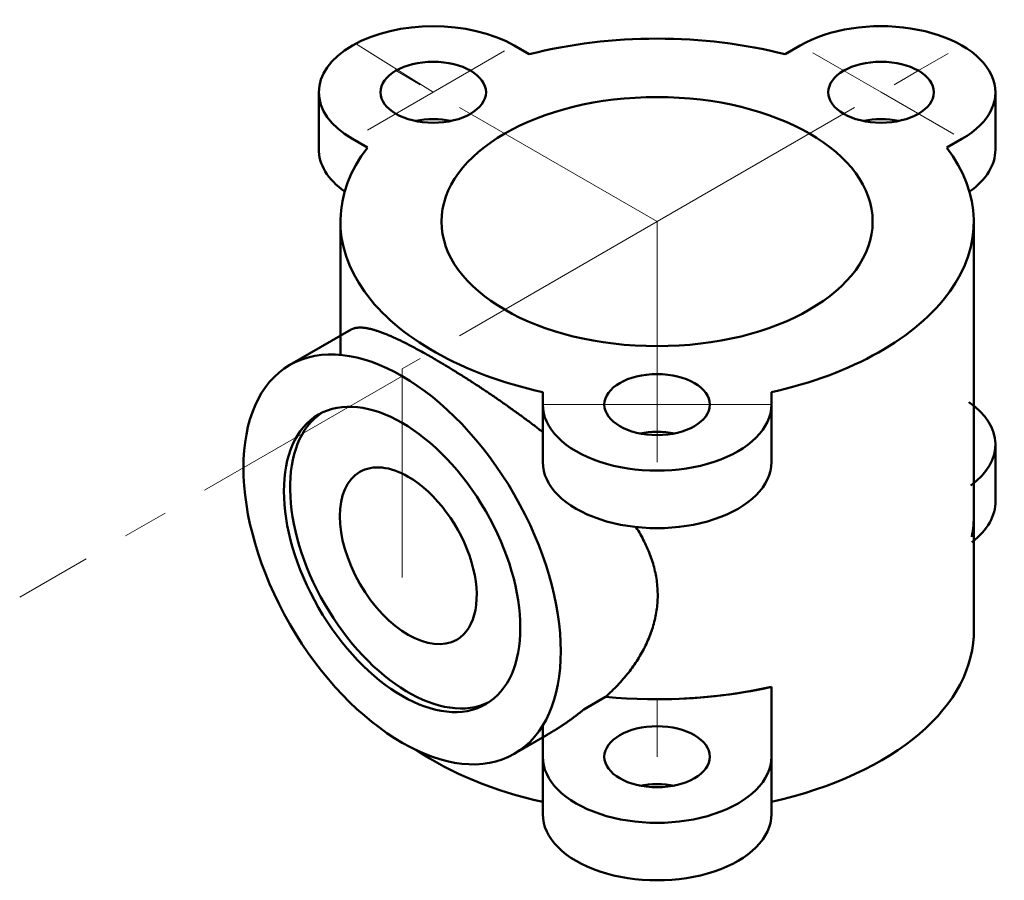
# Model space of a CAD drawing. Units: millimetres. Extents: x 3236 to 3373, y 1300 to 1420.
import ezdxf

# ---------------------------------------------------------------- set-up
doc = ezdxf.new("R2010")
doc.units = ezdxf.units.MM
doc.linetypes.add('CENTER', pattern=[50.8, 31.75, -6.35, 6.35, -6.35])
doc.layers.add('M-CNTR', color=4, linetype='CENTER', lineweight=18)
doc.layers.add('M-OUTL', color=7, linetype='Continuous', lineweight=50)

msp = doc.modelspace()

# ---------------------------------------------------------------- linework, layer by layer
at = {"layer": 'M-CNTR'}
for p, q in [((3293.15, 1409.64), (3282.35, 1416.4)), ((3293.15, 1409.64), (3303.09, 1415.38)), ((3355.5, 1409.64), (3346.02, 1415.11)), ((3360.7, 1412.64), (3364.83, 1415.03)), ((3324.32, 1391.64), (3287.95, 1412.64)), ((3324.32, 1391.64), (3360.7, 1412.64)), ((3293.15, 1409.64), (3283.99, 1404.35)), ((3355.5, 1409.64), (3365.63, 1403.79)), ((3324.32, 1391.64), (3288.82, 1371.14)), ((3324.32, 1366.18), (3324.32, 1391.64)), ((3288.82, 1371.14), (3288.82, 1342.14)), ((3288.82, 1370.14), (3235.58, 1339.4)), ((3340.24, 1366.18), (3308.4, 1366.18)), ((3324.32, 1366.18), (3324.32, 1358.18)), ((3324.32, 1317.18), (3324.32, 1325.18))]:
    msp.add_line(p, q, dxfattribs=at)
at = {"layer": 'M-OUTL'}
for p, q in [((3304.4, 1416.14), (3306.51, 1414.93)), ((3344.24, 1416.14), (3342.14, 1414.93)), ((3277.23, 1401.49), (3277.22, 1409.64)), ((3371.42, 1409.64), (3371.42, 1401.64)), ((3281.89, 1403.14), (3283.99, 1401.93)), ((3366.76, 1403.14), (3364.65, 1401.93)), ((3280.23, 1391.64), (3280.23, 1373.09)), ((3368.41, 1334.64), (3368.41, 1391.64)), ((3273.2, 1371.69), (3281.72, 1376.61)), ((3308.4, 1366.18), (3308.4, 1367.9)), ((3308.4, 1367.9), (3308.4, 1359.9)), ((3340.24, 1366.18), (3340.24, 1367.9)), ((3340.24, 1367.9), (3340.24, 1359.9)), ((3308.4, 1358.18), (3308.4, 1359.9)), ((3340.24, 1358.18), (3340.24, 1359.9)), ((3371.42, 1360.79), (3371.42, 1352.64)), ((3340.24, 1326.9), (3340.24, 1310.9)), ((3314.11, 1323.77), (3317.15, 1325.52)), ((3308.4, 1321.55), (3308.4, 1310.9)), ((3304.43, 1317.59), (3309.01, 1320.24)), ((3308.4, 1309.18), (3308.4, 1310.9)), ((3340.24, 1309.18), (3340.24, 1310.9))]:
    msp.add_line(p, q, dxfattribs=at)
for points in [[(3281.72, 1376.61), (3281.77, 1376.63), (3281.82, 1376.66), (3281.86, 1376.68), (3281.91, 1376.7), (3281.96, 1376.72), (3282.02, 1376.74), (3282.07, 1376.76), (3282.12, 1376.78), (3282.18, 1376.8), (3282.23, 1376.81), (3282.29, 1376.83), (3282.35, 1376.84), (3282.41, 1376.85), (3282.47, 1376.86), (3282.53, 1376.87), (3282.59, 1376.88), (3282.66, 1376.88), (3282.72, 1376.89), (3282.79, 1376.89), (3282.86, 1376.9), (3282.93, 1376.9), (3283, 1376.9), (3283.07, 1376.9), (3283.14, 1376.9), (3283.22, 1376.89), (3283.29, 1376.89), (3283.37, 1376.88), (3283.45, 1376.87), (3283.53, 1376.86), (3283.61, 1376.85), (3283.7, 1376.84), (3283.78, 1376.83), (3283.87, 1376.81), (3283.96, 1376.8), (3284.05, 1376.78), (3284.14, 1376.76), (3284.23, 1376.74), (3284.33, 1376.72), (3284.42, 1376.7), (3284.52, 1376.67), (3284.62, 1376.65), (3284.72, 1376.62), (3284.82, 1376.59), (3284.93, 1376.56), (3285.04, 1376.53), (3285.15, 1376.5), (3285.26, 1376.46), (3285.37, 1376.42), (3285.48, 1376.39), (3285.6, 1376.35), (3285.72, 1376.3), (3285.84, 1376.26), (3285.96, 1376.22), (3286.08, 1376.17), (3286.21, 1376.12), (3286.34, 1376.07), (3286.47, 1376.02), (3286.6, 1375.97), (3286.73, 1375.91), (3286.87, 1375.86), (3287.01, 1375.8), (3287.15, 1375.74), (3287.29, 1375.68), (3287.43, 1375.61), (3287.58, 1375.55), (3287.73, 1375.48), (3287.88, 1375.41), (3288.03, 1375.34), (3288.19, 1375.27), (3288.35, 1375.2), (3288.51, 1375.12), (3288.67, 1375.04), (3288.83, 1374.96), (3289, 1374.88), (3289.17, 1374.8), (3289.34, 1374.71), (3289.51, 1374.62), (3289.68, 1374.54), (3289.86, 1374.44), (3290.04, 1374.35), (3290.22, 1374.26), (3290.4, 1374.16), (3290.58, 1374.06), (3290.77, 1373.96), (3290.96, 1373.86), (3291.15, 1373.76), (3291.34, 1373.66), (3291.54, 1373.55), (3291.73, 1373.44), (3291.93, 1373.33), (3292.13, 1373.22), (3292.33, 1373.11), (3292.53, 1372.99), (3292.73, 1372.88), (3292.94, 1372.76), (3293.15, 1372.64)], [(3293.15, 1372.64), (3293.3, 1372.55), (3293.46, 1372.46), (3293.61, 1372.37), (3293.77, 1372.28), (3293.92, 1372.19), (3294.08, 1372.09), (3294.24, 1372), (3294.4, 1371.91), (3294.56, 1371.81), (3294.72, 1371.72), (3294.88, 1371.62), (3295.04, 1371.52), (3295.2, 1371.42), (3295.36, 1371.33), (3295.52, 1371.23), (3295.69, 1371.13), (3295.85, 1371.03), (3296.01, 1370.93), (3296.18, 1370.83), (3296.34, 1370.72), (3296.5, 1370.62), (3296.67, 1370.52), (3296.83, 1370.42), (3297, 1370.31), (3297.16, 1370.21), (3297.33, 1370.11), (3297.49, 1370), (3297.66, 1369.9), (3297.83, 1369.79), (3297.99, 1369.68), (3298.16, 1369.58), (3298.32, 1369.47), (3298.49, 1369.36), (3298.65, 1369.26), (3298.82, 1369.15), (3298.99, 1369.04), (3299.15, 1368.93), (3299.32, 1368.82), (3299.48, 1368.72), (3299.65, 1368.61), (3299.81, 1368.5), (3299.98, 1368.39), (3300.14, 1368.28), (3300.31, 1368.17), (3300.47, 1368.06), (3300.64, 1367.95), (3300.8, 1367.84), (3300.96, 1367.73), (3301.13, 1367.62), (3301.29, 1367.51), (3301.45, 1367.4), (3301.62, 1367.29), (3301.78, 1367.17), (3301.94, 1367.06), (3302.1, 1366.95), (3302.26, 1366.84), (3302.43, 1366.73), (3302.59, 1366.62), (3302.75, 1366.51), (3302.91, 1366.39), (3303.07, 1366.28), (3303.23, 1366.17), (3303.39, 1366.06), (3303.55, 1365.95), (3303.7, 1365.83), (3303.86, 1365.72), (3304.02, 1365.61), (3304.18, 1365.5), (3304.33, 1365.38), (3304.49, 1365.27), (3304.65, 1365.16), (3304.8, 1365.05), (3304.96, 1364.93), (3305.11, 1364.82), (3305.27, 1364.71), (3305.42, 1364.6), (3305.57, 1364.48), (3305.73, 1364.37), (3305.88, 1364.26), (3306.03, 1364.15), (3306.18, 1364.03), (3306.34, 1363.92), (3306.49, 1363.81), (3306.64, 1363.7), (3306.79, 1363.58), (3306.94, 1363.47), (3307.08, 1363.36), (3307.23, 1363.25), (3307.38, 1363.13), (3307.53, 1363.02), (3307.67, 1362.91), (3307.82, 1362.8), (3307.97, 1362.68), (3308.11, 1362.57), (3308.26, 1362.46), (3308.4, 1362.35)], [(3321.41, 1349.1), (3321.56, 1348.86), (3321.71, 1348.61), (3321.86, 1348.36), (3322, 1348.11), (3322.14, 1347.86), (3322.27, 1347.62), (3322.4, 1347.36), (3322.53, 1347.11), (3322.65, 1346.86), (3322.77, 1346.61), (3322.89, 1346.36), (3323, 1346.1), (3323.11, 1345.85), (3323.21, 1345.6), (3323.31, 1345.34), (3323.41, 1345.09), (3323.5, 1344.83), (3323.59, 1344.57), (3323.67, 1344.31), (3323.75, 1344.06), (3323.82, 1343.8), (3323.89, 1343.54), (3323.96, 1343.28), (3324.02, 1343.02), (3324.08, 1342.76), (3324.13, 1342.5), (3324.18, 1342.24), (3324.22, 1341.97), (3324.26, 1341.71), (3324.29, 1341.45), (3324.32, 1341.19), (3324.35, 1340.93), (3324.37, 1340.66), (3324.38, 1340.4), (3324.39, 1340.14), (3324.4, 1339.87), (3324.4, 1339.61), (3324.4, 1339.35), (3324.39, 1339.08), (3324.37, 1338.82), (3324.36, 1338.56), (3324.33, 1338.29), (3324.31, 1338.03), (3324.28, 1337.77), (3324.24, 1337.51), (3324.2, 1337.25), (3324.15, 1336.99), (3324.1, 1336.73), (3324.05, 1336.47), (3323.99, 1336.21), (3323.92, 1335.95), (3323.86, 1335.69), (3323.78, 1335.43), (3323.71, 1335.17), (3323.63, 1334.92), (3323.54, 1334.66), (3323.45, 1334.41), (3323.36, 1334.15), (3323.26, 1333.9), (3323.16, 1333.65), (3323.05, 1333.4), (3322.94, 1333.15), (3322.83, 1332.9), (3322.71, 1332.65), (3322.59, 1332.41), (3322.46, 1332.16), (3322.33, 1331.92), (3322.2, 1331.68), (3322.06, 1331.44), (3321.92, 1331.2), (3321.78, 1330.96), (3321.63, 1330.72), (3321.48, 1330.49), (3321.33, 1330.25), (3321.17, 1330.02), (3321.01, 1329.79), (3320.85, 1329.56), (3320.68, 1329.33), (3320.51, 1329.11), (3320.34, 1328.88), (3320.16, 1328.66), (3319.98, 1328.44), (3319.8, 1328.22), (3319.61, 1328), (3319.42, 1327.78), (3319.23, 1327.57), (3319.03, 1327.35), (3318.84, 1327.14), (3318.63, 1326.93), (3318.43, 1326.73), (3318.22, 1326.52), (3318.02, 1326.32), (3317.8, 1326.12), (3317.59, 1325.92), (3317.37, 1325.72), (3317.15, 1325.52)], [(3309.01, 1320.24), (3309.07, 1320.27), (3309.13, 1320.31), (3309.19, 1320.34), (3309.25, 1320.38), (3309.31, 1320.41), (3309.36, 1320.44), (3309.42, 1320.48), (3309.48, 1320.51), (3309.54, 1320.55), (3309.6, 1320.58), (3309.65, 1320.62), (3309.71, 1320.65), (3309.77, 1320.69), (3309.83, 1320.72), (3309.88, 1320.75), (3309.94, 1320.79), (3310, 1320.82), (3310.05, 1320.86), (3310.11, 1320.89), (3310.17, 1320.93), (3310.22, 1320.96), (3310.28, 1321), (3310.33, 1321.04), (3310.39, 1321.07), (3310.45, 1321.11), (3310.5, 1321.14), (3310.56, 1321.18), (3310.61, 1321.21), (3310.67, 1321.25), (3310.73, 1321.28), (3310.78, 1321.32), (3310.84, 1321.36), (3310.89, 1321.39), (3310.95, 1321.43), (3311, 1321.46), (3311.06, 1321.5), (3311.11, 1321.54), (3311.16, 1321.57), (3311.22, 1321.61), (3311.27, 1321.65), (3311.33, 1321.68), (3311.38, 1321.72), (3311.43, 1321.75), (3311.49, 1321.79), (3311.54, 1321.83), (3311.6, 1321.86), (3311.65, 1321.9), (3311.7, 1321.94), (3311.76, 1321.97), (3311.81, 1322.01), (3311.86, 1322.05), (3311.91, 1322.09), (3311.97, 1322.12), (3312.02, 1322.16), (3312.07, 1322.2), (3312.12, 1322.23), (3312.18, 1322.27), (3312.23, 1322.31), (3312.28, 1322.35), (3312.33, 1322.38), (3312.38, 1322.42), (3312.44, 1322.46), (3312.49, 1322.5), (3312.54, 1322.53), (3312.59, 1322.57), (3312.64, 1322.61), (3312.69, 1322.65), (3312.74, 1322.69), (3312.79, 1322.72), (3312.84, 1322.76), (3312.89, 1322.8), (3312.94, 1322.84), (3312.99, 1322.88), (3313.04, 1322.91), (3313.09, 1322.95), (3313.14, 1322.99), (3313.19, 1323.03), (3313.24, 1323.07), (3313.29, 1323.11), (3313.34, 1323.15), (3313.39, 1323.18), (3313.44, 1323.22), (3313.49, 1323.26), (3313.54, 1323.3), (3313.59, 1323.34), (3313.64, 1323.38), (3313.68, 1323.42), (3313.73, 1323.46), (3313.78, 1323.5), (3313.83, 1323.53), (3313.88, 1323.57), (3313.92, 1323.61), (3313.97, 1323.65), (3314.02, 1323.69), (3314.07, 1323.73), (3314.11, 1323.77)]]:
    msp.add_lwpolyline(points, dxfattribs=at)
for centre, major_axis, start_param, end_param in [((3293.15, 1409.64), (-15.92, 0), 3.926991, 7.068583), ((3355.5, 1409.64), (-15.92, 0), 2.356129, 5.497853), ((3324.32, 1391.64), (-44.09, 0), 4.29645, 5.128328), ((3293.15, 1401.64), (7.35, 0), 1.230959, 1.910633), ((3355.5, 1401.64), (7.35, 0), 1.230959, 1.910633), ((3293.15, 1401.64), (-15.92, 0), 6.267166, 6.969492), ((3324.32, 1391.64), (-44.09, 0), 5.867246, 7.484523), ((3324.32, 1391.64), (-44.09, 0), 8.223441, 9.840717), ((3355.5, 1401.64), (-15.92, 0), 2.455286, 3.141593), ((3324.32, 1366.18), (-15.92, 0), 6.283185, 9.424778), ((3355.5, 1360.64), (-15.92, 0), 2.471919, 3.835974), ((3289.68, 1345.14), (11.64, -20.15), 3.178817, 6.245961), ((3324.32, 1358.14), (7.35, 0), 1.230959, 1.910633), ((3289.68, 1345.14), (6.74, -11.67), 2.356194, 3.141593), ((3324.32, 1358.18), (-15.92, 0), 6.283185, 9.424778), ((3289.68, 1345.14), (6.74, -11.67), 3.141593, 6.283185), ((3289.68, 1345.14), (6.74, -11.67), 0, 2.356194), ((3355.5, 1352.64), (-15.92, 0), 2.489159, 3.158142), ((3324.32, 1350.64), (-44.09, 0), 9.312433, 9.437132), ((3324.32, 1334.64), (-44.09, 0), 8.223441, 9.437132), ((3324.32, 1350.64), (44.09, 0), 4.549003, 5.081848), ((3324.32, 1350.64), (-44.09, 0), 7.853982, 8.223441), ((3324.32, 1334.64), (-44.09, 0), 6.991466, 7.484523), ((3324.32, 1317.18), (-15.92, 0), 6.283185, 9.424778), ((3324.32, 1309.14), (7.35, 0), 1.230959, 1.910633), ((3324.32, 1309.18), (-15.92, 0), 6.283185, 9.424778)]:
    msp.add_ellipse(centre, major_axis=major_axis, ratio=0.57735, start_param=start_param, end_param=end_param, dxfattribs=at)
for centre, major_axis in [((3293.15, 1409.64), (-7.35, 0)), ((3355.5, 1409.64), (-7.35, 0)), ((3324.32, 1391.64), (-30.01, 0)), ((3288.82, 1344.64), (15.62, -27.05)), ((3324.32, 1366.18), (-7.35, 0)), ((3288.82, 1344.64), (11.64, -20.15)), ((3324.32, 1317.18), (-7.35, 0))]:
    msp.add_ellipse(centre, major_axis=major_axis, ratio=0.57735, dxfattribs=at)

doc.saveas('drawing.dxf')
